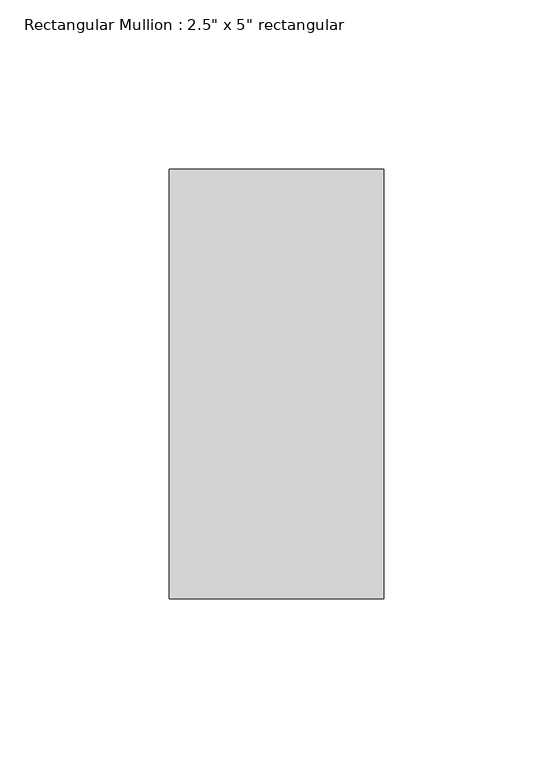
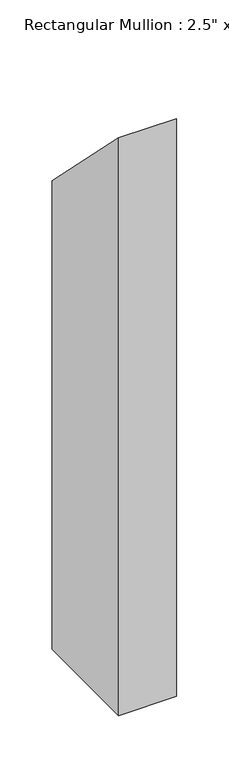
"""IFC4 building model written with IfcOpenShell, lengths in millimetres: member geometry."""

from ifc_helpers import new_model, si_unit, frame, origin, place, context, project, spatial, polyline, outline, extrude, source, transform, mapped, element, save


def member_df81370e(model_context):
    return source(origin(), model_context, "Body", "SweptSolid", [
        extrude(outline(polyline([(-63.5, 63.5), (63.5, -63.5), (63.5, -609.6), (-63.5, -609.6), (-63.5, 63.5)])), frame((-63.5, 0.0, 0.0), z_axis=(1.0, 0.0, 0.0), x_axis=(0.0, 1.0, 0.0)), (0.0, 0.0, 1.0), 63.5),
    ])


if __name__ == "__main__":
    model = new_model("IFC4")
    model_context = context("Model", 3, world=origin())
    ifc_project = project(units=[si_unit("LENGTHUNIT", "METRE", prefix="MILLI")], contexts=[model_context])
    site = spatial("IfcSite", under=ifc_project)
    building = spatial("IfcBuilding", under=site)
    placement = place(None, origin())
    member_shape = member_df81370e(model_context)
    element("IfcMember", 1, ObjectType="Rectangular Mullion : 2.5\" x 5\" rectangular", at=placement, inside=building, context=model_context, shape_type="MappedRepresentation", body=[
        mapped(member_shape, transform((0.0, 0.0, 0.0), x_axis=(1.0, 0.0, 0.0), y_axis=(0.0, 1.0, 0.0), z_axis=(0.0, 0.0, 1.0))),
    ])
    save(model, "model.ifc")

# Revit data of these elements
# Type "Rectangular Mullion : 2.5\" x 5\" rectangular"
#   built-in parameter 1007304 = 0.416667 (stored number, unit not read)
#   built-in parameter 1007301 = 0.104167 (stored number, unit not read)
#   built-in parameter 1007300 = 0.104167 (stored number, unit not read)
# Element 1 (IfcMember, "Rectangular Mullion : 2.5\" x 5\" rectangular")
#   Materials on its faces: "Aluminum"
# Materials
#   "Aluminum": class "Metal", colour RGB 247 247 247, transparency 0, Description = "Aluminum 6061", Cost = 0
